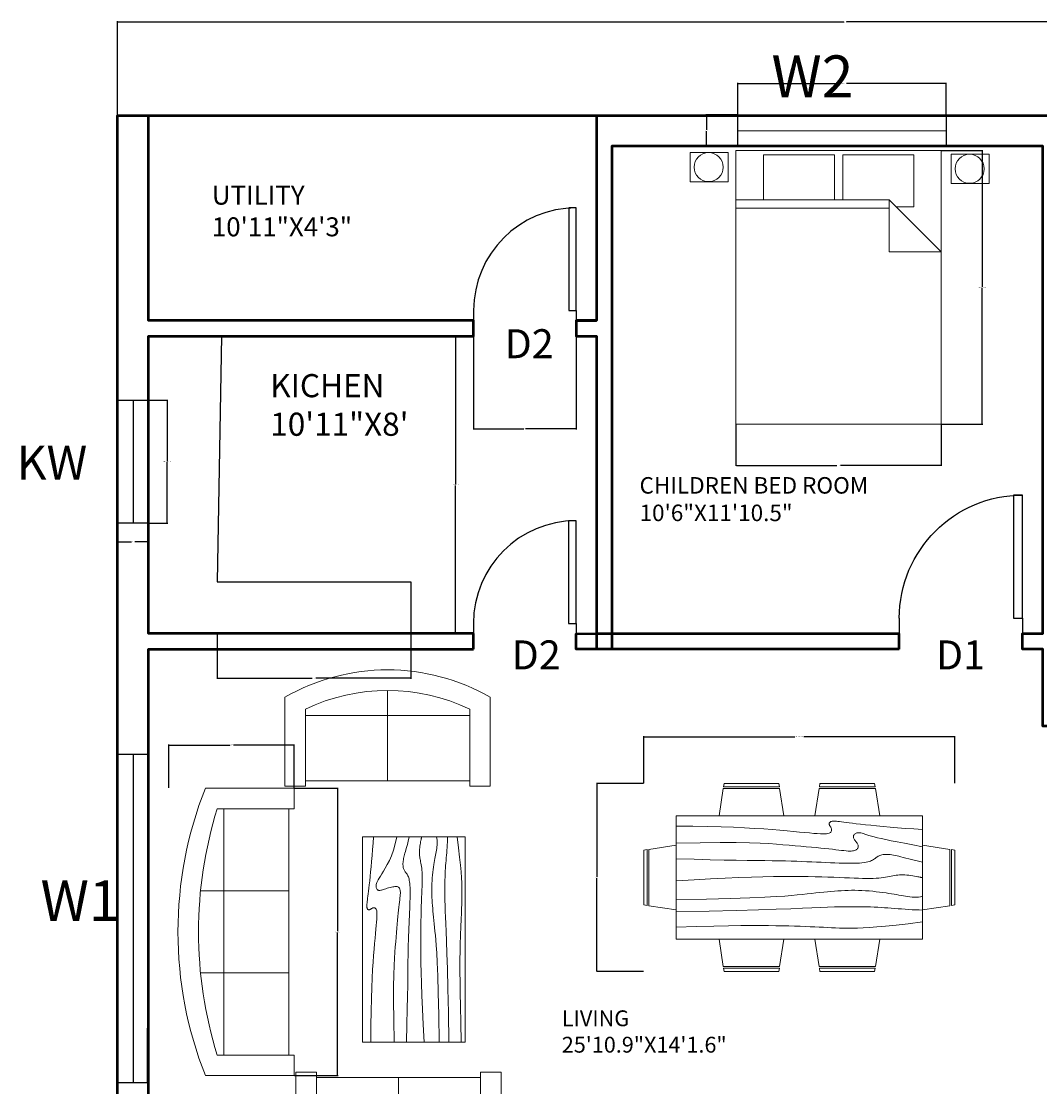
# Model space of a CAD drawing. Units: inches. Extents: x -45 to 1424, y 648 to 1662.
# Tile 6 of 8: x 921 to 1218, y 906 to 1217. Entities that reach past the tile are written whole.
import ezdxf

# ---------------------------------------------------------------- set-up
doc = ezdxf.new("R2010")
doc.units = ezdxf.units.IN
for name, color, linetype, lineweight in [('A-ANNO-DIMS', 2, 'Continuous', 18), ('A-ANNO-TEXT', 7, 'Continuous', 18), ('A-AREA-IDEN', 7, 'Continuous', 18), ('A-FLOR-CASE', 3, 'Continuous', 25), ('DOOR', 2, 'Continuous', 25), ('FURNITURE', 3, 'Continuous', 18), ('WALL', 4, 'Continuous', 50), ('WINDOW', 1, 'Continuous', 25)]:
    doc.layers.add(name, color=color, linetype=linetype, lineweight=lineweight)
doc.styles.get("Standard").update_dxf_attribs({"font": 'arial.ttf'})
doc.dimstyles.get("Standard").update_dxf_attribs({"dimtxt": 0.18, "dimasz": 0.18, "dimexe": 0.18, "dimexo": 0.0625, "dimgap": 0.09, "dimtad": 0, "dimtih": 1, "dimtoh": 1, "dimdec": 4, "dimzin": 0, "dimdsep": 46, "dimtxsty": 'Standard', "dimcen": 0.09, "dimadec": 0, "dimazin": 0, "dimtfac": 1, "dimtdec": 4, "dimtofl": 0, "dimtmove": 0, "dimatfit": 3, "dimfxl": 1, "dimtolj": 1, "dimtzin": 0, "dimarcsym": 0})

# ---------------------------------------------------------------- blocks, each defined once
blk = doc.blocks.new('*U2')
for p, q in [((-24, 0), (-24, -6)), ((0, 0), (0, -6))]:
    blk.add_line(p, q)
blk.add_lwpolyline([(0, 0), (0, 24), (-1.75, 24), (-1.75, 0)], close=True)
blk.add_arc((0, 0), 24, 90, 180)
blk = doc.blocks.new('*U3')
for p, q in [((0, 0), (0, -6)), ((24, 0), (24, -6))]:
    blk.add_line(p, q)
blk.add_lwpolyline([(0, 0), (0, 24), (1.75, 24), (1.75, 0)], close=True)
blk.add_arc((0, 0), 24, 0, 90)
blk = doc.blocks.new('Bed - Queen')
for p, q in [((0, -80.00003), (0, 0)), ((0, 0), (59.99999, 0)), ((59.99999, 0), (59.99999, -80.00003)), ((7.99999, -1.2), (28.79998, -1.2)), ((7.99999, -14.4), (7.99999, -1.2)), ((28.79998, -1.2), (28.79998, -14.4)), ((31.19999, -1.2), (51.99999, -1.2)), ((31.19999, -14.4), (31.19999, -1.2)), ((51.99999, -1.2), (51.99999, -16.4)), ((0, -14.4), (44.8, -14.4)), ((59.99999, -29.6), (44.8, -14.4)), ((44.8, -14.4), (44.8, -29.6)), ((44.8, -16.8), (0, -16.8)), ((51.99999, -16.4), (46.79936, -16.4)), ((44.8, -29.6), (59.99999, -29.6)), ((59.99999, -80.00003), (0, -80.00003))]:
    blk.add_line(p, q)
blk = doc.blocks.new('Sofa - Roundback 7 ft.')
for p, q in [((-12.00002, -32.4421), (-12.00003, -6.5971)), ((11.99997, -32.4421), (11.99998, -6.5971)), ((-36.000027, -34), (-36.000027, -11.4696)), ((35.99998, -34), (35.99998, -11.4696)), ((-35.999844, -13.3819), (35.9998, -13.3819)), ((-36.000027, -32.4421), (35.99998, -32.4421))]:
    blk.add_line(p, q)
for points in [[(-36.000027, -34), (-42.000027, -34), (-42.000027, -8)], [(41.99998, -8), (41.99998, -34), (35.99998, -34)]]:
    blk.add_lwpolyline(points)
for centre, radius, start, end in [((0, -114.25), 114.25, 68.43141, 111.5686), ((-0.00001, -127.1968), 121.1968, 72.72033, 107.2797)]:
    blk.add_arc(centre, radius, start, end)
blk = doc.blocks.new('Sofa - Roundback Loveseat 5 ft.')
for p, q in [((0, -32.44198), (0, -5.99998)), ((-24, -33.99998), (-24, -11.46958)), ((24.00004, -33.99998), (24.00004, -11.46958)), ((-23.9998, -13.38178), (23.99986, -13.38178)), ((-24, -32.44198), (24.00004, -32.44198))]:
    blk.add_line(p, q)
for points in [[(-24, -33.99998), (-30, -33.99998), (-30, -7.99998)], [(30.00004, -7.99998), (30.00004, -33.99998), (24.00004, -33.99998)]]:
    blk.add_lwpolyline(points)
for centre, radius, start, end in [((0, -60.24998), 60.24998, 60.13715, 119.8628), ((0, -61.38438), 55.38444, 64.32083, 115.6792)]:
    blk.add_arc(centre, radius, start, end)
blk = doc.blocks.new('Table - Rectangular Woodgrain 60 x 30 in.')
for p, q in [((0, 0), (0, -30)), ((60, 0), (0, 0)), ((60, -30), (60, 0)), ((0, -30), (60, -30))]:
    blk.add_line(p, q)
for points in [[(0, -2.4), (4.8155, -2.418), (9.0302, -2.4688), (12.709, -2.5477), (15.9167, -2.65), (18.7181, -2.7711), (21.1781, -2.9063), (23.3616, -3.0508), (25.3333, -3.2), (27.1477, -3.3495), (28.8172, -3.4958), (30.3437, -3.636), (31.7291, -3.7667), (32.9756, -3.8849), (34.0849, -3.9875), (35.059, -4.0714), (35.9, -4.1334), (36.6114, -4.1711), (37.2041, -4.1854), (37.6906, -4.1779), (38.0833, -4.15), (38.3948, -4.1034), (38.6375, -4.0396), (38.8239, -3.9602), (38.9666, -3.8667), (39.0764, -3.7608), (39.1573, -3.6448), (39.2116, -3.521), (39.2416, -3.3917), (39.2498, -3.2593), (39.2385, -3.1261), (39.21, -2.9944), (39.1666, -2.8667), (39.111, -2.7447), (39.0468, -2.6281), (38.978, -2.5163), (38.9083, -2.4083), (38.8418, -2.3035), (38.7823, -2.201), (38.7337, -2.1001), (38.7, -2), (38.6844, -1.9003), (38.6875, -1.8021), (38.7094, -1.707), (38.75, -1.6167), (38.8094, -1.5326), (38.8875, -1.4563), (38.9844, -1.3893), (39.1, -1.3333), (39.2351, -1.2896), (39.3937, -1.2583), (39.5804, -1.2396), (39.8, -1.2333), (40.057, -1.2396), (40.3562, -1.2583), (40.7023, -1.2896), (41.1, -1.3333), (41.5547, -1.3895), (42.0755, -1.4573), (42.6721, -1.5361), (43.3542, -1.625), (44.1316, -1.7233), (45.014, -1.8302), (46.0114, -1.9449), (47.1333, -2.0667), (48.3862, -2.1947), (49.7625, -2.3281), (51.2513, -2.4663), (52.8416, -2.6083), (54.5226, -2.7535), (56.2833, -2.9011), (58.1127, -3.0501), (60, -3.2)], [(0, -9.2), (6.5759, -9.0858), (11.9385, -9.0365), (16.2527, -9.0418), (19.6833, -9.0917), (22.3952, -9.1759), (24.5531, -9.2844), (26.322, -9.4069), (27.8666, -9.5333), (29.3241, -9.6553), (30.7203, -9.7719), (32.0532, -9.8837), (33.3208, -9.9917), (34.5213, -10.0965), (35.6526, -10.199), (36.7128, -10.2999), (37.7, -10.4), (38.6129, -10.4996), (39.4531, -10.5969), (40.223, -10.6895), (40.925, -10.775), (41.5613, -10.8512), (42.1344, -10.9156), (42.6465, -10.966), (43.1, -11), (43.4976, -11.0158), (43.8437, -11.0136), (44.143, -10.9942), (44.4, -10.9583), (44.6195, -10.9069), (44.8062, -10.8406), (44.9648, -10.7603), (45.1, -10.6667), (45.2155, -10.5598), (45.3114, -10.4365), (45.3871, -10.2929), (45.4416, -10.125), (45.4743, -9.929), (45.4844, -9.7011), (45.4709, -9.4371), (45.4333, -9.1333), (45.3716, -8.7883), (45.2896, -8.4104), (45.1919, -8.0107), (45.0833, -7.6), (44.9685, -7.1893), (44.8521, -6.7896), (44.7388, -6.4117), (44.6333, -6.0667), (44.54, -5.7628), (44.4614, -5.4979), (44.4001, -5.2675), (44.3583, -5.0667), (44.3384, -4.8909), (44.3427, -4.7354), (44.3736, -4.5956), (44.4333, -4.4667), (44.5236, -4.3453), (44.6427, -4.2333), (44.7884, -4.1339), (44.9583, -4.05), (45.1501, -3.9849), (45.3614, -3.9417), (45.59, -3.9234), (45.8333, -3.9333), (46.0915, -3.9749), (46.3734, -4.0531), (46.6906, -4.1736), (47.0542, -4.3417), (47.4756, -4.5629), (47.9661, -4.8427), (48.5372, -5.1866), (49.2, -5.6), (49.9676, -6.0844), (50.8594, -6.625), (51.8965, -7.2031), (53.1, -7.8), (54.491, -8.3969), (56.0906, -8.975), (57.9199, -9.5156), (60, -10)], [(0, -12.8), (5.1847, -12.9322), (9.6213, -13.0323), (13.3963, -13.1059), (16.5958, -13.1583), (19.3063, -13.1952), (21.614, -13.2219), (23.6054, -13.2439), (25.3666, -13.2667), (26.9728, -13.2947), (28.4531, -13.3281), (29.8256, -13.3663), (31.1083, -13.4083), (32.3191, -13.4535), (33.476, -13.501), (34.597, -13.5501), (35.7, -13.6), (36.7984, -13.6497), (37.8875, -13.6979), (38.9578, -13.743), (40, -13.7833), (41.0047, -13.8174), (41.9625, -13.8438), (42.864, -13.8607), (43.7, -13.8667), (44.4631, -13.8604), (45.1552, -13.8417), (45.7801, -13.8104), (46.3416, -13.7667), (46.8439, -13.7104), (47.2906, -13.6417), (47.6858, -13.5604), (48.0333, -13.4667), (48.3375, -13.3608), (48.6042, -13.2448), (48.8396, -13.121), (49.05, -12.9917), (49.2417, -12.8593), (49.4208, -12.7261), (49.5937, -12.5944), (49.7667, -12.4667), (49.9452, -12.3451), (50.1323, -12.2313), (50.3303, -12.1268), (50.5416, -12.0333), (50.7686, -11.9524), (51.0135, -11.8854), (51.2788, -11.8341), (51.5666, -11.8), (51.8785, -11.7843), (52.2116, -11.7865), (52.562, -11.8059), (52.926, -11.8417), (53.2998, -11.8931), (53.6795, -11.9594), (54.0614, -12.0397), (54.4416, -12.1333), (54.8223, -12.2401), (55.2293, -12.3625), (55.6942, -12.5037), (56.2489, -12.6667), (56.9251, -12.8547), (57.7545, -13.0708), (58.7689, -13.3182), (60, -13.6)], [(0, -18), (5.124, -17.7273), (9.6609, -17.5057), (13.6705, -17.3303), (17.2125, -17.1958), (20.3467, -17.0973), (23.1328, -17.0297), (25.6307, -16.9878), (27.9, -16.9667), (29.9928, -16.9617), (31.9302, -16.9703), (33.7254, -16.9907), (35.3917, -17.0208), (36.9423, -17.0588), (38.3906, -17.1026), (39.7499, -17.1503), (41.0333, -17.2), (42.2519, -17.2496), (43.4073, -17.2969), (44.4986, -17.3395), (45.525, -17.375), (46.4858, -17.4012), (47.3802, -17.4156), (48.2074, -17.416), (48.9667, -17.4), (49.6583, -17.3662), (50.2872, -17.3167), (50.8595, -17.2547), (51.3812, -17.1833), (51.8584, -17.1057), (52.2971, -17.025), (52.7034, -16.9443), (53.0833, -16.8667), (53.443, -16.7951), (53.789, -16.7313), (54.128, -16.6768), (54.4666, -16.6334), (54.8115, -16.6024), (55.1693, -16.5854), (55.5465, -16.5841), (55.95, -16.6), (56.3828, -16.6337), (56.8346, -16.6823), (57.2915, -16.7418), (57.7396, -16.8084), (58.165, -16.878), (58.5539, -16.9469), (58.8924, -17.0111), (59.1666, -17.0667), (59.3679, -17.1107), (59.5078, -17.1438), (59.6032, -17.1675), (59.6708, -17.1833), (59.7275, -17.193), (59.7901, -17.1979), (59.8753, -17.1998), (60, -17.2)], [(0, -22.4), (8.0098, -22.2501), (14.4094, -22.1011), (19.4168, -21.9535), (23.25, -21.8083), (26.1269, -21.6663), (28.2656, -21.5281), (29.884, -21.3947), (31.2, -21.2667), (32.3967, -21.1448), (33.5172, -21.0292), (34.5697, -20.9198), (35.5625, -20.8167), (36.5037, -20.7198), (37.4015, -20.6292), (38.2642, -20.5448), (39.1, -20.4667), (39.9164, -20.3951), (40.7187, -20.3313), (41.5117, -20.2768), (42.3, -20.2333), (43.0883, -20.2024), (43.8812, -20.1854), (44.6836, -20.1841), (45.5, -20.2), (46.3328, -20.234), (47.1747, -20.2844), (48.0163, -20.3488), (48.8479, -20.425), (49.66, -20.5106), (50.4429, -20.6031), (51.1872, -20.7004), (51.8833, -20.8), (52.5246, -20.8999), (53.1166, -20.9995), (53.6681, -21.0983), (54.1875, -21.1958), (54.6834, -21.2919), (55.1646, -21.3859), (55.6394, -21.4777), (56.1167, -21.5667), (56.6028, -21.6515), (57.0961, -21.7266), (57.5929, -21.7852), (58.0896, -21.8208), (58.5823, -21.8268), (59.0674, -21.7964), (59.5412, -21.723), (60, -21.6)], [(0, -25.2), (8.6355, -25.0504), (15.7026, -24.9031), (21.4049, -24.7606), (25.9458, -24.625), (29.529, -24.4988), (32.3578, -24.3844), (34.6359, -24.284), (36.5667, -24.2), (38.3213, -24.1341), (39.9417, -24.0854), (41.437, -24.0523), (42.8167, -24.0333), (44.0901, -24.0268), (45.2667, -24.0313), (46.3557, -24.0451), (47.3667, -24.0667), (48.309, -24.0947), (49.1928, -24.1287), (50.0284, -24.168), (50.826, -24.2125), (51.5959, -24.2617), (52.3483, -24.3151), (53.0935, -24.3725), (53.8417, -24.4334), (54.6009, -24.497), (55.3699, -24.561), (56.1454, -24.6226), (56.9239, -24.6792), (57.7021, -24.7279), (58.4764, -24.7662), (59.2435, -24.7911), (60, -24.8)], [(0, -28.8), (5.6867, -28.6681), (10.45, -28.5698), (14.407, -28.5012), (17.675, -28.4584), (20.3711, -28.4374), (22.6125, -28.4344), (24.5164, -28.4455), (26.2, -28.4667), (27.762, -28.4947), (29.2276, -28.5281), (30.6033, -28.5663), (31.8958, -28.6084), (33.1118, -28.6535), (34.2578, -28.7011), (35.3405, -28.7501), (36.3666, -28.8), (37.3443, -28.8497), (38.288, -28.8974), (39.2137, -28.9412), (40.1375, -28.9792), (41.0753, -29.0093), (42.0432, -29.0297), (43.0572, -29.0384), (44.1333, -29.0333), (45.2936, -29.0114), (46.5843, -28.9641), (48.0579, -28.8816), (49.7666, -28.7542), (51.7629, -28.5721), (54.0989, -28.3255), (56.8272, -28.0048), (60, -27.6)]]:
    blk.add_lwpolyline(points)
blk = doc.blocks.new('Dining Set - 36 x 72 in.')
for p, q in [((-22.2343, 26.00059), (-23.4847, 17.99762)), ((-22.2304, 26), (-5.7608, 26)), ((-22, 27.5), (-22.1562, 26.50042)), ((-5.8416, 26.5), (-22.1534, 26.5)), ((-22, 27.5), (-6, 27.5)), ((-5.8437, 26.49966), (-6, 27.5)), ((-4.5152, 17.99762), (-5.7655, 25.99926)), ((5.7657, 26.00059), (4.5153, 17.99762)), ((5.7696, 26), (22.2392, 26)), ((6, 27.5), (5.8438, 26.50042)), ((22.1584, 26.5), (5.8466, 26.5)), ((6, 27.5), (22, 27.5)), ((22.1563, 26.49966), (22, 27.5)), ((23.4848, 17.99762), (22.2345, 25.99926)), ((36, 18), (-36, 18)), ((-36, 18), (-36, -18)), ((36, -18), (36, 18)), ((-44.0006, 8.23428), (-35.9976, 9.48474)), ((44.0006, 8.23428), (35.9976, 9.48474)), ((-45.5, 8), (-44.5004, 8.15617)), ((-45.5, 8), (-45.5, -8)), ((-44.5, -8.15843), (-44.5, 8.15338)), ((-44, 8.23041), (-44, -8.23915)), ((44, 8.23041), (44, -8.23915)), ((44.5, -8.15843), (44.5, 8.15338)), ((45.5, 8), (44.5005, 8.15617)), ((45.5, 8), (45.5, -8)), ((-44.4997, -8.15631), (-45.5, -8)), ((-35.9976, -9.48476), (-43.9993, -8.2345)), ((35.9976, -9.48476), (43.9993, -8.2345)), ((44.4997, -8.15631), (45.5, -8)), ((-36, -18), (36, -18)), ((-22.2343, -26.0006), (-23.4847, -17.99762)), ((-4.5152, -17.99762), (-5.7655, -25.99928)), ((5.7657, -26.0006), (4.5153, -17.99762)), ((23.4848, -17.99762), (22.2345, -25.99928)), ((-22.2304, -26), (-5.7608, -26)), ((-22, -27.5), (-22.1562, -26.50044)), ((-5.8416, -26.5), (-22.1534, -26.5)), ((-22, -27.5), (-6, -27.5)), ((-5.8437, -26.49967), (-6, -27.5)), ((5.7696, -26), (22.2392, -26)), ((6, -27.5), (5.8438, -26.50044)), ((22.1584, -26.5), (5.8466, -26.5)), ((6, -27.5), (22, -27.5)), ((22.1563, -26.49967), (22, -27.5))]:
    blk.add_line(p, q)
for points in [[(-36, 15), (-31.1772, 14.97754), (-26.8079, 14.91406), (-22.8538, 14.81543), (-19.276, 14.6875), (-16.0362, 14.53613), (-13.0957, 14.36718), (-10.4159, 14.18652), (-7.9583, 14), (-5.6904, 13.81315), (-3.6035, 13.63021), (-1.6954, 13.45508), (0.0365, 13.29166), (1.5945, 13.14388), (2.9811, 13.01562), (4.1988, 12.9108), (5.25, 12.83333), (6.1393, 12.78613), (6.8802, 12.76823), (7.4883, 12.77767), (7.9792, 12.8125), (8.3685, 12.87077), (8.6719, 12.95052), (8.9049, 13.0498), (9.0833, 13.16666), (9.2205, 13.29899), (9.3216, 13.44401), (9.3895, 13.59879), (9.4271, 13.76041), (9.4373, 13.92594), (9.4232, 14.09245), (9.3875, 14.257), (9.3333, 14.41666), (9.2638, 14.56917), (9.1836, 14.71484), (9.0975, 14.85465), (9.0104, 14.98958), (8.9272, 15.1206), (8.8529, 15.2487), (8.7922, 15.37483), (8.75, 15.5), (8.7305, 15.62467), (8.7344, 15.74739), (8.7617, 15.86621), (8.8125, 15.97916), (8.8867, 16.08431), (8.9844, 16.17968), (9.1055, 16.26334), (9.25, 16.33333), (9.4189, 16.38802), (9.6172, 16.42708), (9.8506, 16.45052), (10.125, 16.45833), (10.4463, 16.45052), (10.8203, 16.42708), (11.2529, 16.38802), (11.75, 16.33333), (12.3184, 16.26318), (12.9694, 16.17838), (13.7151, 16.07991), (14.5677, 15.96875), (15.5395, 15.84586), (16.6426, 15.71224), (17.8893, 15.56884), (19.2917, 15.41666), (20.859, 15.25667), (22.5879, 15.08984), (24.4721, 14.91715), (26.5052, 14.73958), (28.6809, 14.5581), (30.9929, 14.3737), (33.4347, 14.18733), (36, 14)], [(-36, 10), (-28.9766, 10.14274), (-23.1725, 10.20442), (-18.4241, 10.19775), (-14.5677, 10.13541), (-11.4399, 10.03011), (-8.877, 9.89453), (-6.7154, 9.74137), (-4.7917, 9.58333), (-2.9698, 9.43082), (-1.2246, 9.28515), (0.4415, 9.14534), (2.026, 9.01041), (3.5266, 8.87939), (4.9408, 8.7513), (6.266, 8.62516), (7.5, 8.5), (8.6411, 8.37549), (9.6914, 8.2539), (10.6538, 8.13818), (11.5312, 8.03125), (12.3267, 7.93603), (13.043, 7.85547), (13.6831, 7.79248), (14.25, 7.75), (14.7471, 7.7303), (15.1797, 7.73307), (15.5537, 7.75732), (15.875, 7.80208), (16.1494, 7.86637), (16.3828, 7.94922), (16.5811, 8.04964), (16.75, 8.16666), (16.8944, 8.29915), (17.0143, 8.44531), (17.1089, 8.60319), (17.1771, 8.77083), (17.218, 8.94629), (17.2305, 9.1276), (17.2137, 9.31282), (17.1667, 9.5), (17.0895, 9.6875), (16.987, 9.875), (16.8649, 10.0625), (16.7292, 10.25), (16.5856, 10.4375), (16.4401, 10.625), (16.2985, 10.8125), (16.1667, 11), (16.05, 11.18733), (15.9518, 11.3737), (15.8752, 11.5581), (15.8229, 11.73958), (15.798, 11.91715), (15.8034, 12.08984), (15.842, 12.25667), (15.9167, 12.41666), (16.0295, 12.56836), (16.1784, 12.70833), (16.3605, 12.83268), (16.5729, 12.9375), (16.8127, 13.01888), (17.0768, 13.07291), (17.3625, 13.0957), (17.6667, 13.08333), (17.9894, 13.03312), (18.3418, 12.94726), (18.7382, 12.82918), (19.1927, 12.68229), (19.7195, 12.51001), (20.3327, 12.31575), (21.0465, 12.10294), (21.875, 11.875), (22.8357, 11.63354), (23.959, 11.37304), (25.2786, 11.08618), (26.8282, 10.76562), (28.6414, 10.40405), (30.752, 9.99414), (33.1936, 9.52856), (36, 9)], [(-36, 5.5), (-30.7157, 5.3348), (-26.069, 5.20963), (-21.9946, 5.11767), (-18.4271, 5.05208), (-15.3009, 5.00602), (-12.5508, 4.97265), (-10.1112, 4.94515), (-7.9167, 4.91666), (-5.909, 4.88167), (-4.0586, 4.83984), (-2.3429, 4.79215), (-0.7396, 4.73958), (0.7739, 4.6831), (2.22, 4.6237), (3.6213, 4.56233), (5, 4.5), (6.373, 4.43782), (7.7344, 4.3776), (9.0723, 4.32129), (10.375, 4.27083), (11.6309, 4.22819), (12.8281, 4.19531), (13.9551, 4.17415), (15, 4.16666), (15.954, 4.17448), (16.819, 4.19791), (17.6001, 4.23698), (18.3021, 4.29166), (18.9299, 4.36198), (19.4883, 4.44791), (19.9823, 4.54948), (20.4167, 4.66666), (20.7969, 4.79899), (21.1302, 4.94401), (21.4245, 5.09879), (21.6875, 5.26041), (21.9271, 5.42594), (22.1511, 5.59245), (22.3672, 5.757), (22.5834, 5.91666), (22.8065, 6.06868), (23.0404, 6.21093), (23.2879, 6.34147), (23.5521, 6.45833), (23.8358, 6.55957), (24.142, 6.64323), (24.4735, 6.70735), (24.8334, 6.75), (25.2235, 6.76969), (25.642, 6.76692), (26.0858, 6.74267), (26.5521, 6.69791), (27.0379, 6.63362), (27.5404, 6.55078), (28.0565, 6.45036), (28.5834, 6.33333), (29.1242, 6.19987), (29.7071, 6.04687), (30.3661, 5.87044), (31.1354, 5.66666), (32.0493, 5.43164), (33.142, 5.16146), (34.4475, 4.85221), (36, 4.5)], [(-36, -1), (-30.7915, -0.6591), (-26.0195, -0.38216), (-21.6519, -0.16284), (-17.6563, 0.00521), (-14.0005, 0.12833), (-10.6523, 0.21289), (-7.5796, 0.26522), (-4.75, 0.29166), (-2.134, 0.29793), (0.2878, 0.28711), (2.5317, 0.26163), (4.6146, 0.22396), (6.5529, 0.17651), (8.3633, 0.12174), (10.0623, 0.06209), (11.6667, 0), (13.1899, -0.06201), (14.6341, -0.1211), (15.9982, -0.17432), (17.2813, -0.21875), (18.4823, -0.25147), (19.6003, -0.26953), (20.6343, -0.27002), (21.5834, -0.25), (22.4481, -0.20768), (23.2357, -0.14584), (23.9549, -0.06836), (24.6146, 0.02083), (25.2235, 0.11784), (25.7904, 0.21875), (26.3241, 0.31966), (26.8334, 0.41666), (27.3265, 0.50618), (27.8099, 0.58593), (28.2894, 0.65397), (28.7709, 0.70833), (29.2601, 0.74707), (29.763, 0.76823), (30.2855, 0.76985), (30.8334, 0.75), (31.4088, 0.70784), (31.9994, 0.64713), (32.589, 0.57275), (33.1615, 0.48958), (33.7008, 0.4025), (34.1908, 0.3164), (34.6153, 0.23616), (34.9584, 0.16666), (35.2099, 0.11165), (35.3848, 0.07031), (35.504, 0.04069), (35.5886, 0.02083), (35.6594, 0.00879), (35.7377, 0.0026), (35.8442, 0.00032), (36, 0)], [(-36, -6.5), (-27.1843, -6.31267), (-20.084, -6.1263), (-14.469, -5.9419), (-10.1094, -5.76042), (-6.7752, -5.58285), (-4.2363, -5.41016), (-2.2629, -5.24333), (-0.625, -5.08334), (0.8708, -4.93099), (2.2715, -4.78646), (3.5872, -4.64974), (4.8281, -4.52084), (6.0046, -4.39974), (7.127, -4.28646), (8.2053, -4.18099), (9.25, -4.08334), (10.2705, -3.99382), (11.2734, -3.91407), (12.2647, -3.84603), (13.25, -3.79167), (14.2354, -3.75293), (15.2266, -3.73177), (16.2295, -3.73015), (17.25, -3.75), (18.2912, -3.79248), (19.3451, -3.85547), (20.4009, -3.93604), (21.4479, -4.03125), (22.4754, -4.13819), (23.4727, -4.25391), (24.4289, -4.37549), (25.3334, -4.5), (26.1785, -4.62492), (26.9694, -4.74935), (27.7145, -4.87281), (28.4219, -4.99479), (29.1, -5.11483), (29.7572, -5.23242), (30.4016, -5.34709), (31.0417, -5.45834), (31.6837, -5.56437), (32.3262, -5.65821), (32.9658, -5.73153), (33.599, -5.77604), (34.2224, -5.78345), (34.8327, -5.74545), (35.4264, -5.65373), (36, -5.5)], [(-36, -10), (-26.4022, -9.81299), (-18.4675, -9.62891), (-11.9839, -9.45069), (-6.7396, -9.28125), (-2.5226, -9.12354), (0.8789, -8.98047), (3.6769, -8.85498), (6.0833, -8.75), (8.2767, -8.66765), (10.3021, -8.60677), (12.1712, -8.56543), (13.8958, -8.54167), (15.4876, -8.53353), (16.9583, -8.53907), (18.3197, -8.55632), (19.5834, -8.58334), (20.7616, -8.61841), (21.8685, -8.66081), (22.9188, -8.71004), (23.9271, -8.76563), (24.9081, -8.82707), (25.8763, -8.89388), (26.8465, -8.96558), (27.8334, -9.04167), (28.8474, -9.12118), (29.8828, -9.20117), (30.93, -9.27824), (31.9792, -9.34896), (33.0205, -9.40991), (34.0443, -9.45768), (35.0407, -9.48885), (36, -9.5)], [(-36, -14.5), (-30.0881, -14.33513), (-25.0332, -14.21224), (-20.7312, -14.12647), (-17.0781, -14.07292), (-13.97, -14.04671), (-11.3027, -14.04297), (-8.9724, -14.05681), (-6.875, -14.08334), (-4.9224, -14.11833), (-3.0905, -14.16016), (-1.3709, -14.20785), (0.2448, -14.26042), (1.7647, -14.3169), (3.1973, -14.3763), (4.5507, -14.43767), (5.8333, -14.5), (7.0554, -14.5621), (8.235, -14.62175), (9.3922, -14.67652), (10.5469, -14.72396), (11.7192, -14.76164), (12.929, -14.78711), (14.1965, -14.79794), (15.5417, -14.79167), (16.9933, -14.76424), (18.6152, -14.70508), (20.4804, -14.60197), (22.6615, -14.44271), (25.2312, -14.21509), (28.2624, -13.9069), (31.8277, -13.50594), (36, -13)]]:
    blk.add_lwpolyline(points)
blk = doc.blocks.new('WIN-W2-BEDROOM-N')
for p, q in [((0, 0), (0, 9)), ((0, 9), (60.88, 9)), ((60.88, 9.18), (60.88, 0)), ((0, 4.5), (60.88, 4.59)), ((60.88, 0), (0, 0))]:
    blk.add_line(p, q)
blk = doc.blocks.new('WIN-KW-KITCHEN')
for p, q in [((0, 36), (9, 36)), ((0, 0), (0, 36)), ((4.5, 36), (4.53, 0)), ((9, 36), (9.05, 0)), ((9.05, 0), (0, 0))]:
    blk.add_line(p, q)
blk = doc.blocks.new('WIN-W1-LIVING')
for p, q in [((0, 96), (9, 96)), ((0, 0), (0, 96)), ((4.5, 96), (4.5, 0)), ((8.72, 0), (9, 96)), ((8.72, 0), (0, 0))]:
    blk.add_line(p, q)
blk = doc.blocks.new('FURN-BEDSIDE-UNIT')
blk.add_lwpolyline([(0, 8.55), (11.15, 8.55), (11.15, 0), (0, 0)], close=True)
blk.add_circle((5.42, 4.31), 4.24)
blk = doc.blocks.new('CASEWORK-KITCHEN')
for p, q in [((1.26, 87), (0, 15.15)), ((0, 15.15), (56.6, 15.15)), ((56.6, 15.15), (56.6, 0))]:
    blk.add_line(p, q)
blk = doc.blocks.new('*D38')
at = {"layer": 'A-ANNO-DIMS', "color": 0, "lineweight": -2, "transparency": 16777216}
for p, q in [((1189.68, 1179.55), (1201.79, 1179.55)), ((1201.61, 1179.37), (1201.61, 1139.74)), ((1201.61, 1099.73), (1201.61, 1139.37)), ((1189.68, 1099.55), (1201.79, 1099.55))]:
    blk.add_line(p, q, dxfattribs=at)
at = {"layer": 'A-ANNO-DIMS', "color": 0, "transparency": 16777216}
for points in [[(1201.58, 1179.37), (1201.64, 1179.37), (1201.61, 1179.55)], [(1201.58, 1099.73), (1201.64, 1099.73), (1201.61, 1099.55)]]:
    blk.add_solid(points, dxfattribs=at)
at = {"layer": 'Defpoints', "color": 0, "transparency": 16777216}
for p in [(1189.61, 1179.55), (1201.61, 1179.55), (1189.61, 1099.55)]:
    blk.add_point(p, dxfattribs=at)
at = {"layer": 'A-ANNO-DIMS', "color": 0, "transparency": 16777216, "insert": (1201.61, 1139.55), "char_height": 0.18, "attachment_point": 5}
blk.add_mtext('\\A1;QUEEN BED 80 TYP.', dxfattribs=at)
blk = doc.blocks.new('*D39')
at = {"layer": 'A-ANNO-DIMS', "color": 0, "lineweight": -2, "transparency": 16777216}
for p, q in [((1129.61, 1099.49), (1129.61, 1087.37)), ((1189.61, 1099.49), (1189.61, 1087.37)), ((1129.79, 1087.55), (1159.09, 1087.55)), ((1189.43, 1087.55), (1160.14, 1087.55))]:
    blk.add_line(p, q, dxfattribs=at)
at = {"layer": 'A-ANNO-DIMS', "color": 0, "transparency": 16777216}
for points in [[(1129.79, 1087.58), (1129.79, 1087.52), (1129.61, 1087.55)], [(1189.43, 1087.58), (1189.43, 1087.52), (1189.61, 1087.55)]]:
    blk.add_solid(points, dxfattribs=at)
at = {"layer": 'Defpoints', "color": 0, "transparency": 16777216}
for p in [(1129.61, 1099.55), (1189.61, 1099.55), (1189.61, 1087.55)]:
    blk.add_point(p, dxfattribs=at)
at = {"layer": 'A-ANNO-DIMS', "color": 0, "transparency": 16777216, "insert": (1159.61, 1087.55), "char_height": 0.18, "attachment_point": 5}
blk.add_mtext('\\A1;60 TYP.', dxfattribs=at)
blk = doc.blocks.new('*D42')
at = {"layer": 'A-ANNO-DIMS', "color": 0, "lineweight": -2, "transparency": 16777216}
for p, q in [((1000.55, 993.17), (1013.27, 993.17)), ((1013.09, 992.99), (1013.09, 951.36)), ((1013.09, 909.35), (1013.09, 950.99)), ((1000.55, 909.17), (1013.27, 909.17))]:
    blk.add_line(p, q, dxfattribs=at)
at = {"layer": 'A-ANNO-DIMS', "color": 0, "transparency": 16777216}
for points in [[(1013.06, 992.99), (1013.12, 992.99), (1013.09, 993.17)], [(1013.06, 909.35), (1013.12, 909.35), (1013.09, 909.17)]]:
    blk.add_solid(points, dxfattribs=at)
at = {"layer": 'Defpoints', "color": 0, "transparency": 16777216}
for p in [(1000.49, 993.17), (1013.09, 993.17), (1000.49, 909.17)]:
    blk.add_point(p, dxfattribs=at)
at = {"layer": 'A-ANNO-DIMS', "color": 0, "transparency": 16777216, "insert": (1013.09, 951.17), "char_height": 0.18, "attachment_point": 5}
blk.add_mtext('\\A1;SOFA 84 TYP.', dxfattribs=at)
blk = doc.blocks.new('*D43')
at = {"layer": 'A-ANNO-DIMS', "color": 0, "lineweight": -2, "transparency": 16777216}
for p, q in [((963.82, 993.24), (963.82, 1005.95)), ((1000.49, 993.24), (1000.49, 1005.95)), ((964, 1005.77), (981.63, 1005.77)), ((1000.31, 1005.77), (982.68, 1005.77))]:
    blk.add_line(p, q, dxfattribs=at)
at = {"layer": 'A-ANNO-DIMS', "color": 0, "transparency": 16777216}
for points in [[(964, 1005.8), (964, 1005.74), (963.82, 1005.77)], [(1000.31, 1005.8), (1000.31, 1005.74), (1000.49, 1005.77)]]:
    blk.add_solid(points, dxfattribs=at)
at = {"layer": 'Defpoints', "color": 0, "transparency": 16777216}
for p in [(963.82, 1005.77), (963.82, 993.17), (1000.49, 993.17)]:
    blk.add_point(p, dxfattribs=at)
at = {"layer": 'A-ANNO-DIMS', "color": 0, "transparency": 16777216, "insert": (982.15, 1005.77), "char_height": 0.18, "attachment_point": 5}
blk.add_mtext('\\A1;37 TYP.', dxfattribs=at)
blk = doc.blocks.new('*D46')
at = {"layer": 'A-ANNO-DIMS', "color": 0, "lineweight": -2, "transparency": 16777216}
for p, q in [((1102.63, 994.63), (1102.63, 1008.39)), ((1102.81, 1008.21), (1146.85, 1008.21)), ((1193.45, 1008.21), (1149.41, 1008.21)), ((1193.63, 994.63), (1193.63, 1008.39))]:
    blk.add_line(p, q, dxfattribs=at)
at = {"layer": 'A-ANNO-DIMS', "color": 0, "transparency": 16777216}
for points in [[(1102.81, 1008.24), (1102.81, 1008.18), (1102.63, 1008.21)], [(1193.45, 1008.24), (1193.45, 1008.18), (1193.63, 1008.21)]]:
    blk.add_solid(points, dxfattribs=at)
at = {"layer": 'Defpoints', "color": 0, "transparency": 16777216}
for p in [(1193.63, 1008.21), (1102.63, 994.56), (1193.63, 994.56)]:
    blk.add_point(p, dxfattribs=at)
at = {"layer": 'A-ANNO-DIMS', "color": 0, "transparency": 16777216, "insert": (1148.13, 1008.21), "char_height": 0.18, "attachment_point": 5}
blk.add_mtext('\\A1;DINING SET 91 TYP.', dxfattribs=at)
blk = doc.blocks.new('*D47')
at = {"layer": 'A-ANNO-DIMS', "color": 0, "lineweight": -2, "transparency": 16777216}
for p, q in [((1102.57, 994.56), (1088.8, 994.56)), ((1088.98, 994.38), (1088.98, 967.24)), ((1088.98, 939.74), (1088.98, 966.88)), ((1102.57, 939.56), (1088.8, 939.56))]:
    blk.add_line(p, q, dxfattribs=at)
at = {"layer": 'A-ANNO-DIMS', "color": 0, "transparency": 16777216}
for points in [[(1088.95, 994.38), (1089.01, 994.38), (1088.98, 994.56)], [(1088.95, 939.74), (1089.01, 939.74), (1088.98, 939.56)]]:
    blk.add_solid(points, dxfattribs=at)
at = {"layer": 'Defpoints', "color": 0, "transparency": 16777216}
for p in [(1088.98, 994.56), (1102.63, 994.56), (1102.63, 939.56)]:
    blk.add_point(p, dxfattribs=at)
at = {"layer": 'A-ANNO-DIMS', "color": 0, "transparency": 16777216, "insert": (1088.98, 967.06), "char_height": 0.18, "attachment_point": 5}
blk.add_mtext('\\A1;55 TYP.', dxfattribs=at)
blk = doc.blocks.new('*D48')
at = {"layer": 'A-ANNO-DIMS', "color": 0, "lineweight": -2, "transparency": 16777216}
for p, q in [((1130.14, 1190.09), (1130.14, 1199.34)), ((1130.32, 1199.16), (1159.23, 1199.16)), ((1190.84, 1199.16), (1161.92, 1199.16)), ((1191.02, 1190.09), (1191.02, 1199.34))]:
    blk.add_line(p, q, dxfattribs=at)
at = {"layer": 'A-ANNO-DIMS', "color": 0, "transparency": 16777216}
for points in [[(1130.32, 1199.19), (1130.32, 1199.13), (1130.14, 1199.16)], [(1190.84, 1199.19), (1190.84, 1199.13), (1191.02, 1199.16)]]:
    blk.add_solid(points, dxfattribs=at)
at = {"layer": 'Defpoints', "color": 0, "transparency": 16777216}
for p in [(1191.02, 1199.16), (1130.14, 1190.03), (1191.02, 1190.03)]:
    blk.add_point(p, dxfattribs=at)
at = {"layer": 'A-ANNO-DIMS', "color": 0, "transparency": 16777216, "insert": (1160.58, 1199.16), "char_height": 0.18, "attachment_point": 5}
blk.add_mtext('\\A1;WINDOW W2 61 TYP.', dxfattribs=at)
blk = doc.blocks.new('*D49')
at = {"layer": 'A-ANNO-DIMS', "color": 0, "lineweight": -2, "transparency": 16777216}
for p, q in [((1130.08, 1190.03), (1120.83, 1190.03)), ((1121.01, 1189.85), (1121.01, 1185.62)), ((1121.01, 1181.03), (1121.01, 1185.25)), ((1130.08, 1180.85), (1120.83, 1180.85))]:
    blk.add_line(p, q, dxfattribs=at)
at = {"layer": 'A-ANNO-DIMS', "color": 0, "transparency": 16777216}
for points in [[(1120.98, 1189.85), (1121.04, 1189.85), (1121.01, 1190.03)], [(1120.98, 1181.03), (1121.04, 1181.03), (1121.01, 1180.85)]]:
    blk.add_solid(points, dxfattribs=at)
at = {"layer": 'Defpoints', "color": 0, "transparency": 16777216}
for p in [(1121.01, 1190.03), (1130.14, 1190.03), (1130.14, 1180.85)]:
    blk.add_point(p, dxfattribs=at)
at = {"layer": 'A-ANNO-DIMS', "color": 0, "transparency": 16777216, "insert": (1121.01, 1185.44), "char_height": 0.18, "attachment_point": 5}
blk.add_mtext('\\A1;9 TYP.', dxfattribs=at)
blk = doc.blocks.new('*D58')
at = {"layer": 'A-ANNO-DIMS', "color": 0, "lineweight": -2, "transparency": 16777216}
for p, q in [((957.97, 1106.64), (963.49, 1106.64)), ((963.31, 1106.46), (963.31, 1088.82)), ((963.31, 1070.82), (963.31, 1088.45)), ((957.97, 1070.64), (963.49, 1070.64))]:
    blk.add_line(p, q, dxfattribs=at)
at = {"layer": 'A-ANNO-DIMS', "color": 0, "transparency": 16777216}
for points in [[(963.28, 1106.46), (963.34, 1106.46), (963.31, 1106.64)], [(963.28, 1070.82), (963.34, 1070.82), (963.31, 1070.64)]]:
    blk.add_solid(points, dxfattribs=at)
at = {"layer": 'Defpoints', "color": 0, "transparency": 16777216}
for p in [(957.91, 1106.64), (963.31, 1106.64), (957.91, 1070.64)]:
    blk.add_point(p, dxfattribs=at)
at = {"layer": 'A-ANNO-DIMS', "color": 0, "transparency": 16777216, "insert": (963.31, 1088.64), "char_height": 0.18, "attachment_point": 5}
blk.add_mtext('\\A1;WINDOW KW 36 TYP.', dxfattribs=at)
blk = doc.blocks.new('*D59')
at = {"layer": 'A-ANNO-DIMS', "color": 0, "lineweight": -2, "transparency": 16777216}
for p, q in [((948.85, 1070.57), (948.85, 1065.06)), ((957.91, 1070.57), (957.91, 1065.06)), ((949.03, 1065.24), (952.92, 1065.24)), ((957.73, 1065.24), (953.84, 1065.24))]:
    blk.add_line(p, q, dxfattribs=at)
at = {"layer": 'A-ANNO-DIMS', "color": 0, "transparency": 16777216}
for points in [[(949.03, 1065.27), (949.03, 1065.21), (948.85, 1065.24)], [(957.73, 1065.27), (957.73, 1065.21), (957.91, 1065.24)]]:
    blk.add_solid(points, dxfattribs=at)
at = {"layer": 'Defpoints', "color": 0, "transparency": 16777216}
for p in [(948.85, 1070.64), (957.91, 1070.64), (957.91, 1065.24)]:
    blk.add_point(p, dxfattribs=at)
at = {"layer": 'A-ANNO-DIMS', "color": 0, "transparency": 16777216, "insert": (953.38, 1065.24), "char_height": 0.18, "attachment_point": 5}
blk.add_mtext('\\A1;9 TYP.', dxfattribs=at)
blk = doc.blocks.new('*D68')
at = {"layer": 'A-ANNO-DIMS', "color": 0, "lineweight": -2, "transparency": 16777216}
for p, q in [((1034.61, 1125.35), (1047.77, 1125.35)), ((1047.59, 1125.17), (1047.59, 1082.03)), ((1047.59, 1038.53), (1047.59, 1081.66)), ((1034.61, 1038.35), (1047.77, 1038.35))]:
    blk.add_line(p, q, dxfattribs=at)
at = {"layer": 'A-ANNO-DIMS', "color": 0, "transparency": 16777216}
for points in [[(1047.56, 1125.17), (1047.62, 1125.17), (1047.59, 1125.35)], [(1047.56, 1038.53), (1047.62, 1038.53), (1047.59, 1038.35)]]:
    blk.add_solid(points, dxfattribs=at)
at = {"layer": 'Defpoints', "color": 0, "transparency": 16777216}
for p in [(1034.54, 1125.35), (1047.59, 1125.35), (1034.54, 1038.35)]:
    blk.add_point(p, dxfattribs=at)
at = {"layer": 'A-ANNO-DIMS', "color": 0, "transparency": 16777216, "insert": (1047.59, 1081.85), "char_height": 0.18, "attachment_point": 5}
blk.add_mtext('\\A1;CASEWORK 87 TYP.', dxfattribs=at)
blk = doc.blocks.new('*D69')
at = {"layer": 'A-ANNO-DIMS', "color": 0, "lineweight": -2, "transparency": 16777216}
for p, q in [((977.94, 1038.29), (977.94, 1025.12)), ((1034.54, 1038.29), (1034.54, 1025.12)), ((978.12, 1025.3), (1005.72, 1025.3)), ((1034.36, 1025.3), (1006.77, 1025.3))]:
    blk.add_line(p, q, dxfattribs=at)
at = {"layer": 'A-ANNO-DIMS', "color": 0, "transparency": 16777216}
for points in [[(978.12, 1025.33), (978.12, 1025.27), (977.94, 1025.3)], [(1034.36, 1025.33), (1034.36, 1025.27), (1034.54, 1025.3)]]:
    blk.add_solid(points, dxfattribs=at)
at = {"layer": 'Defpoints', "color": 0, "transparency": 16777216}
for p in [(977.94, 1038.35), (1034.54, 1038.35), (1034.54, 1025.3)]:
    blk.add_point(p, dxfattribs=at)
at = {"layer": 'A-ANNO-DIMS', "color": 0, "transparency": 16777216, "insert": (1006.24, 1025.3), "char_height": 0.18, "attachment_point": 5}
blk.add_mtext('\\A1;57 TYP.', dxfattribs=at)
blk = doc.blocks.new('*D82')
at = {"layer": 'A-ANNO-DIMS', "color": 0, "lineweight": -2, "transparency": 16777216}
for p, q in [((948.85, 1189.91), (948.85, 1217.36)), ((949.03, 1217.18), (1161.16, 1217.18)), ((1374.07, 1217.18), (1161.95, 1217.18)), ((1374.25, 1189.91), (1374.25, 1217.36))]:
    blk.add_line(p, q, dxfattribs=at)
at = {"layer": 'A-ANNO-DIMS', "color": 0, "transparency": 16777216}
for points in [[(949.03, 1217.21), (949.03, 1217.15), (948.85, 1217.18)], [(1374.07, 1217.21), (1374.07, 1217.15), (1374.25, 1217.18)]]:
    blk.add_solid(points, dxfattribs=at)
at = {"layer": 'Defpoints', "color": 0, "transparency": 16777216}
for p in [(1374.25, 1217.18), (948.85, 1189.85), (1374.25, 1189.85)]:
    blk.add_point(p, dxfattribs=at)
at = {"layer": 'A-ANNO-DIMS', "color": 0, "transparency": 16777216, "insert": (1161.55, 1217.18), "char_height": 0.18, "attachment_point": 5}
blk.add_mtext('\\A1;425.4', dxfattribs=at)
blk = doc.blocks.new('*D94')
at = {"layer": 'A-ANNO-DIMS', "color": 0, "lineweight": -2, "transparency": 16777216}
for p, q in [((1052.86, 1125.29), (1052.86, 1098.02)), ((1082.85, 1125.29), (1082.85, 1098.02)), ((1053.04, 1098.2), (1067.64, 1098.2)), ((1082.67, 1098.2), (1068.07, 1098.2))]:
    blk.add_line(p, q, dxfattribs=at)
at = {"layer": 'A-ANNO-DIMS', "color": 0, "transparency": 16777216}
for points in [[(1053.04, 1098.23), (1053.04, 1098.17), (1052.86, 1098.2)], [(1082.67, 1098.23), (1082.67, 1098.17), (1082.85, 1098.2)]]:
    blk.add_solid(points, dxfattribs=at)
at = {"layer": 'Defpoints', "color": 0, "transparency": 16777216}
for p in [(1052.86, 1125.35), (1082.85, 1125.35), (1052.86, 1098.2)]:
    blk.add_point(p, dxfattribs=at)
at = {"layer": 'A-ANNO-DIMS', "color": 0, "transparency": 16777216, "insert": (1067.86, 1098.2), "char_height": 0.18, "attachment_point": 5}
blk.add_mtext('\\A1;30', dxfattribs=at)

msp = doc.modelspace()

# ---------------------------------------------------------------- linework, layer by layer
at = {"layer": 'WALL'}
for p, q in [((1082.8541, 1129.8478), (1088.8541, 1129.8478)), ((1052.8542, 1033.8478), (1052.8542, 1038.3478)), ((1177.3544, 1033.8478), (1177.3544, 1038.3478))]:
    msp.add_line(p, q, dxfattribs=at)
msp.add_lwpolyline([(1374.2541, 1189.8478), (1374.2541, 721.8478), (948.8541, 721.8478), (948.8541, 1189.8478)], close=True, dxfattribs=at)
for points in [[(1052.8542, 1038.3478), (957.8541, 1038.3478), (957.8541, 1125.3478), (1052.8562, 1125.3478), (1052.8562, 1129.8478), (957.8541, 1129.8478), (957.8541, 1189.8478)], [(1088.8541, 1189.8478), (1088.8541, 1129.8478), (1082.8541, 1129.8639), (1082.8541, 1125.3478), (1088.8541, 1125.3478), (1088.8541, 1033.8478)], [(1229.8512, 1011.3478), (1219.3541, 1011.3478), (1219.3541, 1033.8478), (1213.3544, 1033.8478), (1213.3544, 1038.3478), (1219.3541, 1038.3478), (1219.3541, 1180.8478), (1093.3541, 1180.8478), (1093.3541, 1033.8478)], [(1177.3544, 1033.8478), (1082.8542, 1033.8478), (1082.8542, 1038.3144), (1088.8541, 1038.3478), (1177.3544, 1038.3478)], [(1188.7541, 721.8478), (1188.7541, 730.8478), (1188.5825, 784.14), (1179.7541, 784.14), (1179.7541, 730.8478), (957.8541, 730.8478), (957.8541, 859.7478), (1137.7546, 859.7478), (1137.7546, 864.2478), (957.8541, 864.2478), (957.8541, 1033.8478), (1052.8542, 1033.8478)]]:
    msp.add_lwpolyline(points, dxfattribs=at)

# ---------------------------------------------------------------- block references
at = {"layer": 'A-FLOR-CASE'}
msp.add_blockref('CASEWORK-KITCHEN', (977.9441, 1038.3478), dxfattribs=at)
at = {"layer": 'DOOR'}
for name, p, xscale, yscale, zscale in [('*U2', (1082.9111, 1132.8319), 1.25, 1.25, 1.25), ('*U3', (1213.3544, 1042.8478), -1.5, 1.5, 1.5), ('*U2', (1082.8542, 1041.3478), 1.25, 1.25, 1.25)]:
    msp.add_blockref(name, p, dxfattribs=dict(at, xscale=xscale, yscale=yscale, zscale=zscale))
at = {"layer": 'FURNITURE'}
for name, p in [('FURN-BEDSIDE-UNIT', (1116.1961, 1170.4148)), ('Bed - Queen', (1129.6137, 1179.5539)), ('FURN-BEDSIDE-UNIT', (1192.4928, 1169.9271)), ('Sofa - Roundback Loveseat 5 ft.', (1027.7591, 1027.7648)), ('Dining Set - 36 x 72 in.', (1148.1311, 967.0634))]:
    msp.add_blockref(name, p, dxfattribs=at)
for name, p, rotation in [('Sofa - Roundback 7 ft.', (966.4877, 951.1743), 89.99999549093542), ('Table - Rectangular Woodgrain 60 x 30 in.', (1020.4757, 918.9475), 89.99999999999976), ('Sofa - Roundback Loveseat 5 ft.', (1030.9343, 876.1746), 180)]:
    msp.add_blockref(name, p, dxfattribs=dict(at, rotation=rotation))
at = {"layer": 'WINDOW'}
for name, p in [('WIN-W2-BEDROOM-N', (1130.1381, 1180.8478)), ('WIN-KW-KITCHEN', (948.8541, 1070.6378)), ('WIN-W1-LIVING', (948.8541, 907.0818))]:
    msp.add_blockref(name, p, dxfattribs=at)

# ---------------------------------------------------------------- texts
at = {"layer": 'A-ANNO-TEXT', "insert": (1139.9848, 1207.3833), "char_height": 12.26218, "width": 1.05025, "attachment_point": 1}
msp.add_mtext('W2', dxfattribs=at)
at = {"layer": 'A-ANNO-TEXT', "attachment_point": 1}
for s, width, gutter_width, heights, insert, char_height in [('D2', 4.069942, 42.3777, [0], (1061.9518, 1127.3435), 8.47554), ('KW', 23.512637, 49.6518, [9.9304], (919.321, 1093.3145), 9.93036), ('D2', 4.069942, 42.3777, [0], (1064.0022, 1036.3782), 8.47554), ('D1', 8.475535, 42.3777, [0], (1188.0423, 1036.3782), 8.47554), ('W1', 18.68524, 59.1031, [0], (926.3038, 966.2139), 11.82062)]:
    msp.add_mtext_dynamic_manual_height_columns(s, width=width, gutter_width=gutter_width, heights=heights, dxfattribs=dict(at, insert=insert, char_height=char_height))
at = {"layer": 'A-AREA-IDEN', "attachment_point": 1}
for s, width, gutter_width, insert, char_height in [('UTILITY\\P10\'11"X4\'3"', 7.386172, 26.803, (976.3868, 1169.3181), 5.556295), ('LIVING\\P25\'10.9"X14\'1.6"', 4.630949, 23.1547, (1078.6974, 928.2245), 4.630949)]:
    msp.add_mtext_dynamic_manual_height_columns(s, width=width, gutter_width=gutter_width, heights=[0], dxfattribs=dict(at, insert=insert, char_height=char_height))
for s, insert, char_height in [('KICHEN\\P10\'11"X8\'', (993.4661, 1114.2264), 6.76397), ('CHILDREN BED ROOM\\P10\'6"X11\'10.5"', (1101.4193, 1084.1146), 4.825426)]:
    msp.add_mtext(s, dxfattribs=dict(at, insert=insert, char_height=char_height))

# ---------------------------------------------------------------- dimensions: what is measured, and where the dimension line sits
at = {"layer": 'A-ANNO-DIMS'}
dim = msp.add_linear_dim(base=(1374.2541, 1217.1757), p1=(948.8541, 1189.8478), p2=(1374.2541, 1189.8478), dimstyle='Standard', override={"dimdec": 1, "dimlfac": 1, "dimrnd": 0, "dimzin": 0, "dimdsep": 46, "dimlunit": 2}, dxfattribs=at)
dim.commit()
dim.dimension.update_dxf_attribs({"geometry": '*D82', "text_midpoint": (1161.5541, 1217.1757)})
for base, p1, p2, text, picture, middle in [((1191.0154, 1199.1573), (1130.1382, 1190.0257), (1191.0154, 1190.0257), 'WINDOW W2 <> TYP.', '*D48', (1160.5768, 1199.1573)), ((1189.6137, 1087.5538), (1129.6137, 1099.5538), (1189.6137, 1099.5538), '<> TYP.', '*D39', (1159.6137, 1087.5538)), ((957.9087, 1065.2374), (948.8541, 1070.6374), (957.9087, 1070.6374), '<> TYP.', '*D59', (953.3814, 1065.2374)), ((1034.5433, 1025.2978), (977.9446, 1038.3478), (1034.5433, 1038.3478), '<> TYP.', '*D69', (1006.2439, 1025.2978)), ((1193.6311, 1008.2134), (1102.6311, 994.5634), (1193.6311, 994.5634), 'DINING SET <> TYP.', '*D46', (1148.1311, 1008.2134))]:
    dim = msp.add_linear_dim(base=base, p1=p1, p2=p2, text=text, dimstyle='Standard', override={"dimdec": 0, "dimlfac": 1, "dimrnd": 0, "dimzin": 0, "dimdsep": 46, "dimlunit": 2}, dxfattribs=at)
    dim.commit()
    dim.dimension.update_dxf_attribs({"geometry": picture, "text_midpoint": middle})
for base, p1, p2, angle, text, picture, middle in [((1121.0067, 1190.0257), (1130.1382, 1180.8478), (1130.1382, 1190.0257), 90, '<> TYP.', '*D49', (1121.0067, 1185.4367)), ((1201.6137, 1179.5539), (1189.6137, 1099.5538), (1189.6137, 1179.5539), 90, 'QUEEN BED <> TYP.', '*D38', (1201.6137, 1139.5539)), ((1047.5933, 1125.3478), (1034.5433, 1038.3478), (1034.5433, 1125.3478), 90, 'CASEWORK <> TYP.', '*D68', (1047.5933, 1081.8478)), ((963.3087, 1106.6374), (957.9087, 1070.6374), (957.9087, 1106.6374), 90, 'WINDOW KW <> TYP.', '*D58', (963.3087, 1088.6374)), ((963.821, 1005.7743), (1000.4877, 993.1743), (963.821, 993.1743), 179.999995, '<> TYP.', '*D43', (982.1543, 1005.7743)), ((1088.9811, 994.5634), (1102.6311, 939.5634), (1102.6311, 994.5634), 90, '<> TYP.', '*D47', (1088.9811, 967.0634)), ((1013.0877, 993.1743), (1000.4877, 909.1743), (1000.4877, 993.1743), 89.999995, 'SOFA <> TYP.', '*D42', (1013.0877, 951.1743))]:
    dim = msp.add_linear_dim(base=base, p1=p1, p2=p2, angle=angle, text=text, dimstyle='Standard', override={"dimdec": 0, "dimlfac": 1, "dimrnd": 0, "dimzin": 0, "dimdsep": 46, "dimlunit": 2}, dxfattribs=at)
    dim.commit()
    dim.dimension.update_dxf_attribs({"geometry": picture, "text_midpoint": middle})
dim = msp.add_linear_dim(base=(1052.8562, 1098.1978), p1=(1082.8541, 1125.3478), p2=(1052.8562, 1125.3478), angle=180, dimstyle='Standard', override={"dimdec": 0, "dimlfac": 1, "dimrnd": 0, "dimzin": 0, "dimdsep": 46, "dimlunit": 2}, dxfattribs=at)
dim.commit()
dim.dimension.update_dxf_attribs({"geometry": '*D94', "text_midpoint": (1067.8552, 1098.1978)})

doc.saveas('drawing.dxf')
